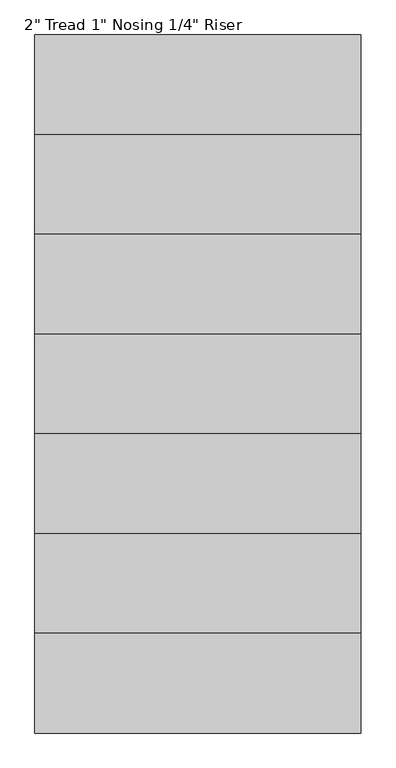
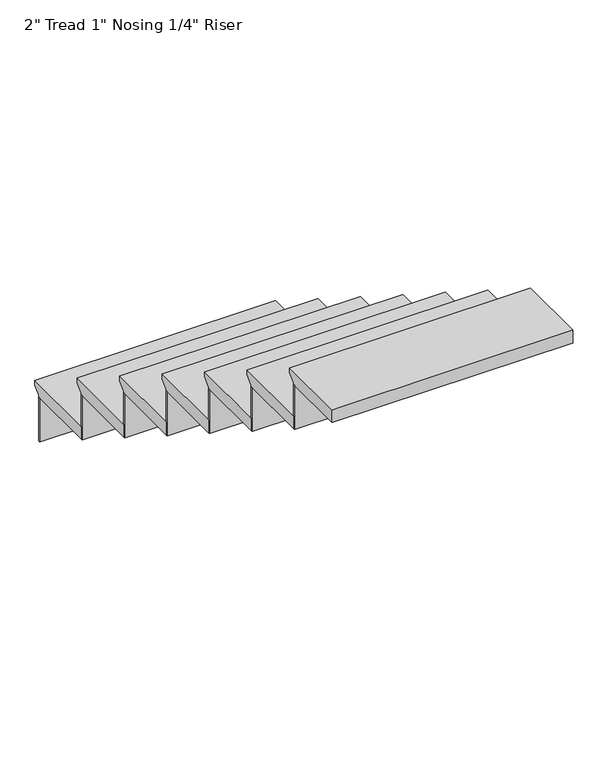
"""IFC4 building model written with IfcOpenShell, lengths in millimetres: stair flight geometry."""

from ifc_helpers import new_model, si_unit, frame, origin, place, context, project, spatial, polyline, outline, extrude, source, transform, mapped, element, save


def stair_flight_95b2deb1(model_context):
    return source(origin(), model_context, "Body", "SweptSolid", [
        extrude(outline(polyline([(494.0027016, 5765.8), (798.8027016, 5765.8), (798.8027016, 5746.75), (773.4027016, 5721.35), (773.4027016, 5715.0), (494.0027016, 5715.0), (494.0027016, 5765.8)])), frame((8683.6260838, 0.0, 0.0), z_axis=(1.0, 0.0, 0.0), x_axis=(0.0, 1.0, 0.0)), (0.0, 0.0, 1.0), 914.4),
        extrude(outline(polyline([(8683.6260838, 767.0527016), (8683.6260838, 773.4027016), (9598.0260838, 773.4027016), (9598.0260838, 767.0527016), (8683.6260838, 767.0527016)])), frame((0.0, 0.0, 5537.2), z_axis=(0.0, 0.0, 1.0), x_axis=(1.0, 0.0, 0.0)), (0.0, 0.0, 1.0), 177.8),
        extrude(outline(polyline([(8683.6260838, 487.6527016), (8683.6260838, 494.0027016), (9598.0260838, 494.0027016), (9598.0260838, 487.6527016), (8683.6260838, 487.6527016)])), frame((0.0, 0.0, 5715.0), z_axis=(0.0, 0.0, 1.0), x_axis=(1.0, 0.0, 0.0)), (0.0, 0.0, 1.0), 177.8),
        extrude(outline(polyline([(214.6027016, 5943.6), (519.4027016, 5943.6), (519.4027016, 5924.55), (494.0027016, 5899.15), (494.0027016, 5892.8), (214.6027016, 5892.8), (214.6027016, 5943.6)])), frame((8683.6260838, 0.0, 0.0), z_axis=(1.0, 0.0, 0.0), x_axis=(0.0, 1.0, 0.0)), (0.0, 0.0, 1.0), 914.4),
        extrude(outline(polyline([(8683.6260838, 208.2527016), (8683.6260838, 214.6027016), (9598.0260838, 214.6027016), (9598.0260838, 208.2527016), (8683.6260838, 208.2527016)])), frame((0.0, 0.0, 5892.8), z_axis=(0.0, 0.0, 1.0), x_axis=(1.0, 0.0, 0.0)), (0.0, 0.0, 1.0), 177.8),
        extrude(outline(polyline([(-64.7972984, 6121.4), (240.0027016, 6121.4), (240.0027016, 6102.35), (214.6027016, 6076.95), (214.6027016, 6070.6), (-64.7972984, 6070.6), (-64.7972984, 6121.4)])), frame((8683.6260838, 0.0, 0.0), z_axis=(1.0, 0.0, 0.0), x_axis=(0.0, 1.0, 0.0)), (0.0, 0.0, 1.0), 914.4),
        extrude(outline(polyline([(8683.6260838, -71.1472984), (8683.6260838, -64.7972984), (9598.0260838, -64.7972984), (9598.0260838, -71.1472984), (8683.6260838, -71.1472984)])), frame((0.0, 0.0, 6070.6), z_axis=(0.0, 0.0, 1.0), x_axis=(1.0, 0.0, 0.0)), (0.0, 0.0, 1.0), 177.8),
        extrude(outline(polyline([(-344.1972984, 6299.2), (-39.3972984, 6299.2), (-39.3972984, 6280.15), (-64.7972984, 6254.75), (-64.7972984, 6248.4), (-344.1972984, 6248.4), (-344.1972984, 6299.2)])), frame((8683.6260838, 0.0, 0.0), z_axis=(1.0, 0.0, 0.0), x_axis=(0.0, 1.0, 0.0)), (0.0, 0.0, 1.0), 914.4),
        extrude(outline(polyline([(8683.6260838, -350.5472984), (8683.6260838, -344.1972984), (9598.0260838, -344.1972984), (9598.0260838, -350.5472984), (8683.6260838, -350.5472984)])), frame((0.0, 0.0, 6248.4), z_axis=(0.0, 0.0, 1.0), x_axis=(1.0, 0.0, 0.0)), (0.0, 0.0, 1.0), 177.8),
        extrude(outline(polyline([(-623.5972984, 6477.0), (-318.7972984, 6477.0), (-318.7972984, 6457.95), (-344.1972984, 6432.55), (-344.1972984, 6426.2), (-623.5972984, 6426.2), (-623.5972984, 6477.0)])), frame((8683.6260838, 0.0, 0.0), z_axis=(1.0, 0.0, 0.0), x_axis=(0.0, 1.0, 0.0)), (0.0, 0.0, 1.0), 914.4),
        extrude(outline(polyline([(8683.6260838, -629.9472984), (8683.6260838, -623.5972984), (9598.0260838, -623.5972984), (9598.0260838, -629.9472984), (8683.6260838, -629.9472984)])), frame((0.0, 0.0, 6426.2), z_axis=(0.0, 0.0, 1.0), x_axis=(1.0, 0.0, 0.0)), (0.0, 0.0, 1.0), 177.8),
        extrude(outline(polyline([(-902.9972984, 6654.8), (-598.1972984, 6654.8), (-598.1972984, 6635.75), (-623.5972984, 6610.35), (-623.5972984, 6604.0), (-902.9972984, 6604.0), (-902.9972984, 6654.8)])), frame((8683.6260838, 0.0, 0.0), z_axis=(1.0, 0.0, 0.0), x_axis=(0.0, 1.0, 0.0)), (0.0, 0.0, 1.0), 914.4),
        extrude(outline(polyline([(8683.6260838, -909.3472984), (8683.6260838, -902.9972984), (9598.0260838, -902.9972984), (9598.0260838, -909.3472984), (8683.6260838, -909.3472984)])), frame((0.0, 0.0, 6604.0), z_axis=(0.0, 0.0, 1.0), x_axis=(1.0, 0.0, 0.0)), (0.0, 0.0, 1.0), 177.8),
        extrude(outline(polyline([(-1156.9972984, 6832.6), (-877.5972984, 6832.6), (-877.5972984, 6813.55), (-902.9972984, 6788.15), (-902.9972984, 6781.8), (-1156.9972984, 6781.8), (-1156.9972984, 6832.6)])), frame((8683.6260838, 0.0, 0.0), z_axis=(1.0, 0.0, 0.0), x_axis=(0.0, 1.0, 0.0)), (0.0, 0.0, 1.0), 914.4),
    ])


if __name__ == "__main__":
    model = new_model("IFC4")
    model_context = context("Model", 3, world=origin())
    ifc_project = project(units=[si_unit("LENGTHUNIT", "METRE", prefix="MILLI")], contexts=[model_context])
    site = spatial("IfcSite", under=ifc_project)
    building = spatial("IfcBuilding", under=site)
    placement = place(None, origin())
    stair_flight_shape = stair_flight_95b2deb1(model_context)
    element("IfcStairFlight", 1, ObjectType="2\" Tread 1\" Nosing 1/4\" Riser", at=placement, inside=building, context=model_context, shape_type="MappedRepresentation", body=[
        mapped(stair_flight_shape, transform((0.0, 0.0, 0.0), x_axis=(1.0, 0.0, 0.0), y_axis=(0.0, 1.0, 0.0), z_axis=(0.0, 0.0, 1.0))),
    ])
    save(model, "model.ifc")
